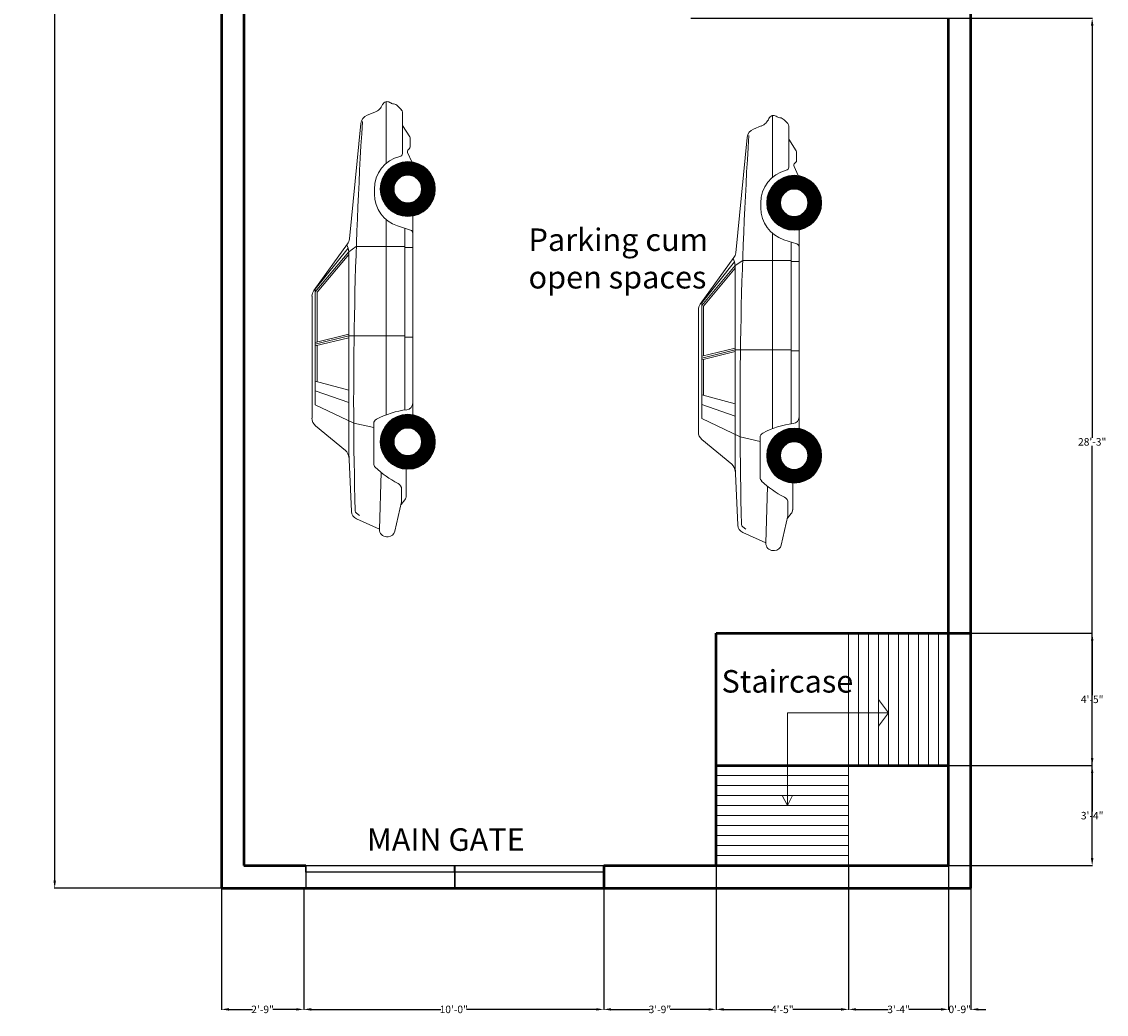
# Model space of a CAD drawing. Units: inches. Extents: x -250 to 2650, y 180 to 1183.
# Tile 1 of 10: x -250 to 184, y 180 to 577. Entities that reach past the tile are written whole.
import ezdxf

# ---------------------------------------------------------------- set-up
doc = ezdxf.new("R2010")
doc.units = ezdxf.units.IN
doc.header["$MEASUREMENT"] = 0
for name, color, linetype, lineweight in [('A-ANNO-DIMS', 2, 'Continuous', 18), ('A-AREA-IDEN', 3, 'Continuous', 18), ('A-DOOR', 4, 'Continuous', 25), ('A-EQPM', 8, 'Continuous', 18), ('A-FLOR-STRS', 8, 'Continuous', 18), ('A-WALL', 7, 'Continuous', 50)]:
    doc.layers.add(name, color=color, linetype=linetype, lineweight=lineweight)
doc.styles.get("Standard").update_dxf_attribs({"font": 'arial.ttf'})
doc.dimstyles.get("Standard").update_dxf_attribs({"dimtxt": 3, "dimasz": 3, "dimexe": 0.18, "dimexo": 0.0625, "dimgap": 0.09, "dimtad": 0, "dimtih": 1, "dimtoh": 1, "dimdec": 0, "dimzin": 0, "dimdsep": 46, "dimlunit": 3, "dimtxsty": 'Standard', "dimcen": 0.09, "dimadec": 0, "dimazin": 0, "dimtfac": 1, "dimtdec": 0, "dimtofl": 0, "dimtmove": 0, "dimatfit": 3, "dimfxl": 1, "dimtolj": 1, "dimtzin": 0, "dimarcsym": 0})

# ---------------------------------------------------------------- blocks, each defined once
blk = doc.blocks.new('*U3')
for p, q in [((0, 0), (0, -6)), ((40, 0), (40, -6))]:
    blk.add_line(p, q)
blk.add_lwpolyline([(0, 0), (40, 0), (40, -1.75), (0, -1.75)], close=True)
blk = doc.blocks.new('Car - sedan  side')
for p, q in [((-139.53, 35.99), (-129.64, 47.91)), ((-128.57, 32.64), (-121.22, 48.02)), ((-77.81, 49.34), (-126.58, 49.34)), ((-74.7, 48.02), (-121.22, 48.02)), ((-120.32, 34.67), (-115.67, 48.02)), ((-115.4, 34.67), (-111.74, 48.02)), ((-94.41, 34.67), (-97.73, 48.02)), ((-93.72, 34.67), (-97.04, 48.02)), ((-93.03, 34.67), (-96.34, 48.02)), ((-60.02, 34.65), (-76.07, 48.02)), ((-56.87, 35.13), (-75.48, 48.59)), ((-58.54, 34.93), (-74.99, 48.02)), ((-97.55, 47.3), (-111.94, 47.3)), ((-76.26, 47.3), (-96.16, 47.3)), ((-61.08, 34.66), (-76.26, 47.3)), ((-60.02, 34.65), (-58.54, 34.93)), ((-57.21, 35.38), (-58.54, 34.93)), ((-170.93, 22.32), (-166.81, 31.56)), ((-164.57, 31.6), (-165.48, 30.35)), ((-140.23, 34.67), (-163.88, 33.56)), ((-62.28, 34.67), (-140.23, 34.67)), ((-130.39, 24.63), (-128.57, 32.64)), ((-93.72, 19.62), (-93.72, 34.67)), ((-62.28, 34.67), (-60.02, 34.65)), ((-57.97, 31.61), (-60.02, 34.65)), ((-57.97, 19.62), (-57.97, 31.61)), ((-54.93, 34.4), (-8.75, 29.8)), ((-4.21, 24.18), (-5.42, 27.27)), ((-148.26, 21.7), (-171.11, 22.33)), ((-128.78, 24.63), (-144.79, 24.63)), ((-36.97, 24.38), (-34.94, 24.38)), ((-174, 19.51), (-174, 18.91)), ((-47.2, 19.62), (-125.23, 19.62)), ((-93.72, 12.14), (-93.72, 19.62)), ((-57.97, 12.14), (-57.97, 19.62)), ((0, 19.62), (-24.7, 19.62)), ((-160.12, 13.48), (-171.81, 16.16)), ((-159.22, 12.14), (-161.08, 13.7)), ((-155.01, 13.48), (-160.12, 13.48)), ((-51.4, 9.89), (-49.69, 15.14)), ((-4.23, 13.19), (-20.72, 13.19)), ((-9.5, 13.19), (-14.1, 10.2)), ((-3.22, 13.59), (-1.77, 14.97)), ((-147.03, 11.6), (-157.73, 11.6)), ((-120.62, 9.03), (-125.23, 9.03)), ((-50.67, 12.14), (-123.32, 12.14)), ((-45.76, 9.03), (-120.62, 9.03)), ((-94.21, 9.03), (-94.21, 12.14)), ((-58.39, 9.03), (-58.39, 12.14)), ((-20.36, 11.06), (-24.06, 9.44)), ((-18.83, 10.42), (-19.11, 10.76)), ((-14.68, 10.03), (-18.01, 10.03))]:
    blk.add_line(p, q)
at = {"const_width": 5.49}
for points in [[(-127.8, 11, -1), (-144.3, 11, -1)], [(-26.69, 11, -1), (-43.19, 11, -1)]]:
    blk.add_lwpolyline(points, format="xyb", close=True, dxfattribs=at)
for centre, radius in [((-136.05, 11), 11), ((-34.94, 11), 11), ((-136.05, 11), 5.51), ((-34.94, 11), 5.51)]:
    blk.add_circle(centre, radius)
for centre, radius, start, end in [((-126.58, 45.38), 3.97, 90, 140.3029), ((-77.81, 45.38), 3.97, 54.135, 90), ((-142.58, 38.53), 3.97, 272.6827, 320.3029), ((-54.54, 38.35), 3.97, 234.135, 264.3123), ((-163.72, 30.18), 3.38, 92.6827, 155.9736), ((-163.62, 30.91), 1.17, 91.491, 143.9553), ((-118.51, -1702.12), 1734.79, 86.34698, 91.49105), ((-9.15, 25.82), 4, 21.3107, 84.3123), ((-171.18, 19.51), 2.82, 88.4193, 180), ((-118.09, -2.78), 38.85, 136.3964, 152.9097), ((-144.79, 22.64), 1.98, 90, 136.3964), ((-128.78, 22.64), 1.98, 28.1371, 90), ((-157.14, 7.48), 34.14, 6.5135, 28.1371), ((-36.97, 11), 13.38, 90, 161.9732), ((-34.94, 11), 13.38, 13.5864, 90), ((0.9, 26.18), 5.49, 201.3107, 247.7048), ((-171.18, 18.91), 2.82, 180, 257.0905), ((-1.92, 19.3), 1.94, 325.3744, 67.7048), ((2.46, 16.28), 3.37, 145.3744, 172.3839), ((-155.01, 16.1), 2.62, 270, 332.9097), ((-20.72, 14.43), 1.24, 193.5864, 270), ((-4.23, 14.65), 1.46, 270, 313.7173), ((-3.82, 17.12), 2.96, 313.7173, 352.3839), ((-157.73, 13.93), 2.32, 230.1291, 270), ((-120.62, 11.65), 2.62, 186.5135, 270), ((-52.58, 10.27), 1.24, 270, 341.9732), ((-19.93, 10.09), 1.06, 39.301, 113.7159), ((-18.01, 11.09), 1.06, 219.301, 270), ((-14.68, 11.09), 1.06, 270, 303.047)]:
    blk.add_arc(centre, radius, start, end)
blk = doc.blocks.new('*D14')
at = {"layer": 'A-ANNO-DIMS', "color": 0, "lineweight": -2, "transparency": 16777216}
for p, q in [((-170.03, 1070.02), (-236.85, 1070.02)), ((-236.67, 1067.02), (-236.67, 657.77)), ((-236.67, 233.02), (-236.67, 642.28)), ((-170.03, 230.02), (-236.85, 230.02))]:
    blk.add_line(p, q, dxfattribs=at)
at = {"layer": 'A-ANNO-DIMS', "color": 0, "transparency": 16777216}
for points in [[(-237.17, 1067.02), (-236.17, 1067.02), (-236.67, 1070.02)], [(-237.17, 233.02), (-236.17, 233.02), (-236.67, 230.02)]]:
    blk.add_solid(points, dxfattribs=at)
at = {"layer": 'Defpoints', "color": 0, "transparency": 16777216}
for p in [(-169.97, 1070.02), (-236.67, 230.02), (-169.97, 230.02)]:
    blk.add_point(p, dxfattribs=at)
at = {"layer": 'A-ANNO-DIMS', "color": 0, "transparency": 16777216, "insert": (-236.67, 650.02), "char_height": 3, "attachment_point": 5}
blk.add_mtext("\\A1;{\\H5x;70'}", dxfattribs=at)
blk = doc.blocks.new('*D58')
at = {"layer": 'A-ANNO-DIMS', "color": 0, "lineweight": -2, "transparency": 16777216}
for p, q in [((17.87, 578.02), (178.71, 578.02)), ((178.53, 575.02), (178.53, 410.15)), ((178.53, 242.02), (178.53, 406.9)), ((-160.91, 239.02), (178.71, 239.02))]:
    blk.add_line(p, q, dxfattribs=at)
at = {"layer": 'A-ANNO-DIMS', "color": 0, "transparency": 16777216}
for points in [[(178.03, 575.02), (179.03, 575.02), (178.53, 578.02)], [(178.03, 242.02), (179.03, 242.02), (178.53, 239.02)]]:
    blk.add_solid(points, dxfattribs=at)
at = {"layer": 'Defpoints', "color": 0, "transparency": 16777216}
for p in [(17.8, 578.02), (-160.97, 239.02), (178.53, 239.02)]:
    blk.add_point(p, dxfattribs=at)
at = {"layer": 'A-ANNO-DIMS', "color": 0, "transparency": 16777216, "insert": (178.53, 408.52), "char_height": 3, "attachment_point": 5}
blk.add_mtext('\\A1;28\'-3"', dxfattribs=at)
blk = doc.blocks.new('*D60')
at = {"layer": 'A-ANNO-DIMS', "color": 0, "lineweight": -2, "transparency": 16777216}
for p, q in [((-169.97, 229.96), (-169.97, 181.34)), ((-136.97, 229.96), (-136.97, 181.34)), ((-166.97, 181.52), (-157.57, 181.52)), ((-139.97, 181.52), (-149.37, 181.52))]:
    blk.add_line(p, q, dxfattribs=at)
at = {"layer": 'A-ANNO-DIMS', "color": 0, "transparency": 16777216}
for points in [[(-166.97, 182.02), (-166.97, 181.02), (-169.97, 181.52)], [(-139.97, 182.02), (-139.97, 181.02), (-136.97, 181.52)]]:
    blk.add_solid(points, dxfattribs=at)
at = {"layer": 'Defpoints', "color": 0, "transparency": 16777216}
for p in [(-169.97, 230.02), (-136.97, 230.02), (-136.97, 181.52)]:
    blk.add_point(p, dxfattribs=at)
at = {"layer": 'A-ANNO-DIMS', "color": 0, "transparency": 16777216, "insert": (-153.47, 181.52), "char_height": 3, "attachment_point": 5}
blk.add_mtext('\\A1;2\'-9"', dxfattribs=at)
blk = doc.blocks.new('*D61')
at = {"layer": 'A-ANNO-DIMS', "color": 0, "lineweight": -2, "transparency": 16777216}
for p, q in [((-136.97, 229.96), (-136.97, 181.34)), ((-16.97, 229.96), (-16.97, 181.34)), ((-133.97, 181.52), (-82.07, 181.52)), ((-19.97, 181.52), (-71.87, 181.52))]:
    blk.add_line(p, q, dxfattribs=at)
at = {"layer": 'A-ANNO-DIMS', "color": 0, "transparency": 16777216}
for points in [[(-133.97, 182.02), (-133.97, 181.02), (-136.97, 181.52)], [(-19.97, 182.02), (-19.97, 181.02), (-16.97, 181.52)]]:
    blk.add_solid(points, dxfattribs=at)
at = {"layer": 'Defpoints', "color": 0, "transparency": 16777216}
for p in [(-136.97, 230.02), (-16.97, 230.02), (-16.97, 181.52)]:
    blk.add_point(p, dxfattribs=at)
at = {"layer": 'A-ANNO-DIMS', "color": 0, "transparency": 16777216, "insert": (-76.97, 181.52), "char_height": 3, "attachment_point": 5}
blk.add_mtext('\\A1;10\'-0"', dxfattribs=at)
blk = doc.blocks.new('*D62')
at = {"layer": 'A-ANNO-DIMS', "color": 0, "lineweight": -2, "transparency": 16777216}
for p, q in [((28.03, 238.96), (28.03, 181.34)), ((-16.97, 229.96), (-16.97, 181.34)), ((-13.97, 181.52), (1.45, 181.52)), ((25.03, 181.52), (9.61, 181.52))]:
    blk.add_line(p, q, dxfattribs=at)
at = {"layer": 'A-ANNO-DIMS', "color": 0, "transparency": 16777216}
for points in [[(-13.97, 182.02), (-13.97, 181.02), (-16.97, 181.52)], [(25.03, 182.02), (25.03, 181.02), (28.03, 181.52)]]:
    blk.add_solid(points, dxfattribs=at)
at = {"layer": 'Defpoints', "color": 0, "transparency": 16777216}
for p in [(28.03, 239.02), (-16.97, 230.02), (28.03, 181.52)]:
    blk.add_point(p, dxfattribs=at)
at = {"layer": 'A-ANNO-DIMS', "color": 0, "transparency": 16777216, "insert": (5.53, 181.52), "char_height": 3, "attachment_point": 5}
blk.add_mtext('\\A1;3\'-9"', dxfattribs=at)
blk = doc.blocks.new('*D63')
at = {"layer": 'A-ANNO-DIMS', "color": 0, "lineweight": -2, "transparency": 16777216}
for p, q in [((28.03, 238.96), (28.03, 181.34)), ((81.03, 238.96), (81.03, 181.34)), ((31.03, 181.52), (50.39, 181.52)), ((78.03, 181.52), (58.67, 181.52))]:
    blk.add_line(p, q, dxfattribs=at)
at = {"layer": 'A-ANNO-DIMS', "color": 0, "transparency": 16777216}
for points in [[(31.03, 182.02), (31.03, 181.02), (28.03, 181.52)], [(78.03, 182.02), (78.03, 181.02), (81.03, 181.52)]]:
    blk.add_solid(points, dxfattribs=at)
at = {"layer": 'Defpoints', "color": 0, "transparency": 16777216}
for p in [(28.03, 239.02), (81.03, 239.02), (81.03, 181.52)]:
    blk.add_point(p, dxfattribs=at)
at = {"layer": 'A-ANNO-DIMS', "color": 0, "transparency": 16777216, "insert": (54.53, 181.52), "char_height": 3, "attachment_point": 5}
blk.add_mtext('\\A1;4\'-5"', dxfattribs=at)
blk = doc.blocks.new('*D64')
at = {"layer": 'A-ANNO-DIMS', "color": 0, "lineweight": -2, "transparency": 16777216}
for p, q in [((81.03, 238.96), (81.03, 181.34)), ((121.03, 238.96), (121.03, 181.34)), ((84.03, 181.52), (96.95, 181.52)), ((118.03, 181.52), (105.11, 181.52))]:
    blk.add_line(p, q, dxfattribs=at)
at = {"layer": 'A-ANNO-DIMS', "color": 0, "transparency": 16777216}
for points in [[(84.03, 182.02), (84.03, 181.02), (81.03, 181.52)], [(118.03, 182.02), (118.03, 181.02), (121.03, 181.52)]]:
    blk.add_solid(points, dxfattribs=at)
at = {"layer": 'Defpoints', "color": 0, "transparency": 16777216}
for p in [(81.03, 239.02), (121.03, 239.02), (121.03, 181.52)]:
    blk.add_point(p, dxfattribs=at)
at = {"layer": 'A-ANNO-DIMS', "color": 0, "transparency": 16777216, "insert": (101.03, 181.52), "char_height": 3, "attachment_point": 5}
blk.add_mtext('\\A1;3\'-4"', dxfattribs=at)
blk = doc.blocks.new('*D65')
at = {"layer": 'A-ANNO-DIMS', "color": 0, "lineweight": -2, "transparency": 16777216}
for p, q in [((121.02886, 238.962048), (121.02886, 181.344548)), ((130.02886, 229.962048), (130.02886, 181.344548)), ((118.02886, 181.524548), (115.02886, 181.524548)), ((133.02886, 181.524548), (136.02886, 181.524548))]:
    blk.add_line(p, q, dxfattribs=at)
at = {"layer": 'A-ANNO-DIMS', "color": 0, "transparency": 16777216}
for points in [[(118.02886, 182.024548), (118.02886, 181.024548), (121.02886, 181.524548)], [(133.02886, 182.024548), (133.02886, 181.024548), (130.02886, 181.524548)]]:
    blk.add_solid(points, dxfattribs=at)
at = {"layer": 'Defpoints', "color": 0, "transparency": 16777216}
for p in [(121.02886, 239.024548), (130.02886, 230.024548), (130.02886, 181.524548)]:
    blk.add_point(p, dxfattribs=at)
at = {"layer": 'A-ANNO-DIMS', "color": 0, "transparency": 16777216, "insert": (125.52886, 181.524548), "char_height": 3, "attachment_point": 5}
blk.add_mtext('\\A1;0\'-9"', dxfattribs=at)
blk = doc.blocks.new('*D66')
at = {"layer": 'A-ANNO-DIMS', "color": 0, "lineweight": -2, "transparency": 16777216}
for p, q in [((121.09, 279.02), (178.71, 279.02)), ((178.53, 276.02), (178.53, 260.65)), ((178.53, 242.02), (178.53, 257.4)), ((121.09, 239.02), (178.71, 239.02))]:
    blk.add_line(p, q, dxfattribs=at)
at = {"layer": 'A-ANNO-DIMS', "color": 0, "transparency": 16777216}
for points in [[(178.03, 276.02), (179.03, 276.02), (178.53, 279.02)], [(178.03, 242.02), (179.03, 242.02), (178.53, 239.02)]]:
    blk.add_solid(points, dxfattribs=at)
at = {"layer": 'Defpoints', "color": 0, "transparency": 16777216}
for p in [(121.03, 279.02), (178.53, 279.02), (121.03, 239.02)]:
    blk.add_point(p, dxfattribs=at)
at = {"layer": 'A-ANNO-DIMS', "color": 0, "transparency": 16777216, "insert": (178.53, 259.02), "char_height": 3, "attachment_point": 5}
blk.add_mtext('\\A1;3\'-4"', dxfattribs=at)
blk = doc.blocks.new('*D67')
at = {"layer": 'A-ANNO-DIMS', "color": 0, "lineweight": -2, "transparency": 16777216}
for p, q in [((121.09, 332.02), (178.71, 332.02)), ((178.53, 329.02), (178.53, 307.14)), ((178.53, 282.02), (178.53, 303.91)), ((121.09, 279.02), (178.71, 279.02))]:
    blk.add_line(p, q, dxfattribs=at)
at = {"layer": 'A-ANNO-DIMS', "color": 0, "transparency": 16777216}
for points in [[(178.03, 329.02), (179.03, 329.02), (178.53, 332.02)], [(178.03, 282.02), (179.03, 282.02), (178.53, 279.02)]]:
    blk.add_solid(points, dxfattribs=at)
at = {"layer": 'Defpoints', "color": 0, "transparency": 16777216}
for p in [(121.03, 332.02), (178.53, 332.02), (121.03, 279.02)]:
    blk.add_point(p, dxfattribs=at)
at = {"layer": 'A-ANNO-DIMS', "color": 0, "transparency": 16777216, "insert": (178.53, 305.52), "char_height": 3, "attachment_point": 5}
blk.add_mtext('\\A1;4\'-5"', dxfattribs=at)

msp = doc.modelspace()

# ---------------------------------------------------------------- linework, layer by layer
at = {"layer": 'A-FLOR-STRS'}
for p, q in [((81.03, 239.02), (81.03, 332.02)), ((85.03, 279.02), (85.03, 332.02)), ((89.03, 279.02), (89.03, 332.02)), ((93.03, 279.02), (93.03, 332.02)), ((97.03, 279.02), (97.03, 332.02)), ((101.03, 279.02), (101.03, 332.02)), ((105.03, 279.02), (105.03, 332.02)), ((109.03, 279.02), (109.03, 332.02)), ((113.03, 279.02), (113.03, 332.02)), ((117.03, 279.02), (117.03, 332.02)), ((97.03, 300.14), (93.03, 305.52)), ((56.54, 300.14), (56.54, 263.02)), ((56.54, 300.14), (97.03, 300.14)), ((97.03, 300.14), (93.03, 294.75)), ((28.03, 275.02), (81.03, 275.02)), ((28.03, 271.02), (81.03, 271.02)), ((28.03, 267.02), (81.03, 267.02)), ((56.54, 263.02), (54.53, 267.02)), ((56.54, 263.02), (58.55, 267.02)), ((28.03, 263.02), (81.03, 263.02)), ((28.03, 259.02), (81.03, 259.02)), ((28.03, 255.02), (81.03, 255.02)), ((28.03, 251.02), (81.03, 251.02)), ((28.03, 247.02), (81.03, 247.02)), ((28.03, 243.02), (81.03, 243.02))]:
    msp.add_line(p, q, dxfattribs=at)
at = {"layer": 'A-WALL'}
for p, q in [((-169.97, 1070.02), (-169.97, 230.02)), ((130.03, 230.02), (130.03, 1070.02)), ((-160.97, 1061.02), (-160.97, 239.02)), ((121.03, 332.02), (121.03, 578.02)), ((28.03, 332.02), (130.03, 332.02)), ((28.03, 239.02), (28.03, 332.02)), ((121.03, 239.02), (121.03, 332.02)), ((28.03, 279.02), (121.03, 279.02)), ((-160.97, 239.02), (-136.22, 239.02)), ((-16.97, 239.02), (121.03, 239.02)), ((-16.97, 239.02), (-16.97, 230.02)), ((-169.97, 230.02), (-136.97, 230.02)), ((-169.97, 230.02), (130.03, 230.02))]:
    msp.add_line(p, q, dxfattribs=at)

# ---------------------------------------------------------------- block references
at = {"layer": 'A-DOOR', "xscale": 1.490620935821662, "yscale": 1.490620935821662, "zscale": 1.490620935821662}
for p in [(-136.22, 239.02), (-76.6, 239.02)]:
    msp.add_blockref('*U3', p, dxfattribs=at)
at = {"layer": 'A-EQPM', "rotation": 90}
for p in [(-84.35, 544.6), (70.27, 539.08)]:
    msp.add_blockref('Car - sedan  side', p, dxfattribs=at)

# ---------------------------------------------------------------- texts
at = {"layer": 'A-AREA-IDEN', "char_height": 9, "attachment_point": 1}
for s, width, insert in [('Parking cum open spaces ', 87.4783, (-47.04, 493.88)), ('Staircase  ', 87.4783, (30.2, 317.24)), ('MAIN GATE ', 78.0851, (-111.74, 253.94))]:
    msp.add_mtext_dynamic_manual_height_columns(s, width=width, gutter_width=1, heights=[0], dxfattribs=dict(at, insert=insert))

# ---------------------------------------------------------------- dimensions: what is measured, and where the dimension line sits
at = {"layer": 'A-ANNO-DIMS'}
dim = msp.add_linear_dim(base=(-236.67, 230.02), p1=(-169.97, 1070.02), p2=(-169.97, 230.02), angle=90, text='{\\H5x;<>}', dimstyle='Standard', override={"dimclrd": 0, "dimclre": 0, "dimclrt": 0}, dxfattribs=at)
dim.commit()
dim.dimension.update_dxf_attribs({"geometry": '*D14', "text_midpoint": (-236.67, 650.02)})
for base, p1, p2, picture, middle in [((178.53, 239.02), (17.8, 578.02), (-160.97, 239.02), '*D58', (178.53, 408.52)), ((178.53, 332.02), (121.03, 279.02), (121.03, 332.02), '*D67', (178.53, 305.52)), ((178.53, 279.02), (121.03, 239.02), (121.03, 279.02), '*D66', (178.53, 259.02))]:
    dim = msp.add_linear_dim(base=base, p1=p1, p2=p2, angle=90, dimstyle='Standard', override={"dimdec": 1, "dimlfac": 1, "dimrnd": 0, "dimzin": 1, "dimdsep": 46, "dimlunit": 4, "dimfrac": 2}, dxfattribs=at)
    dim.commit()
    dim.dimension.update_dxf_attribs({"geometry": picture, "text_midpoint": middle})
for base, p1, p2, picture, middle in [((28.03, 181.52), (-16.97, 230.02), (28.03, 239.02), '*D62', (5.53, 181.52)), ((81.03, 181.52), (28.03, 239.02), (81.03, 239.02), '*D63', (54.53, 181.52)), ((121.03, 181.52), (81.03, 239.02), (121.03, 239.02), '*D64', (101.03, 181.52)), ((130.03, 181.52), (121.03, 239.02), (130.03, 230.02), '*D65', (125.53, 181.52)), ((-136.97, 181.52), (-169.97, 230.02), (-136.97, 230.02), '*D60', (-153.47, 181.52)), ((-16.97, 181.52), (-136.97, 230.02), (-16.97, 230.02), '*D61', (-76.97, 181.52))]:
    dim = msp.add_linear_dim(base=base, p1=p1, p2=p2, dimstyle='Standard', override={"dimdec": 1, "dimlfac": 1, "dimrnd": 0, "dimzin": 1, "dimdsep": 46, "dimlunit": 4, "dimfrac": 2}, dxfattribs=at)
    dim.commit()
    dim.dimension.update_dxf_attribs({"geometry": picture, "text_midpoint": middle})

doc.saveas('drawing.dxf')
